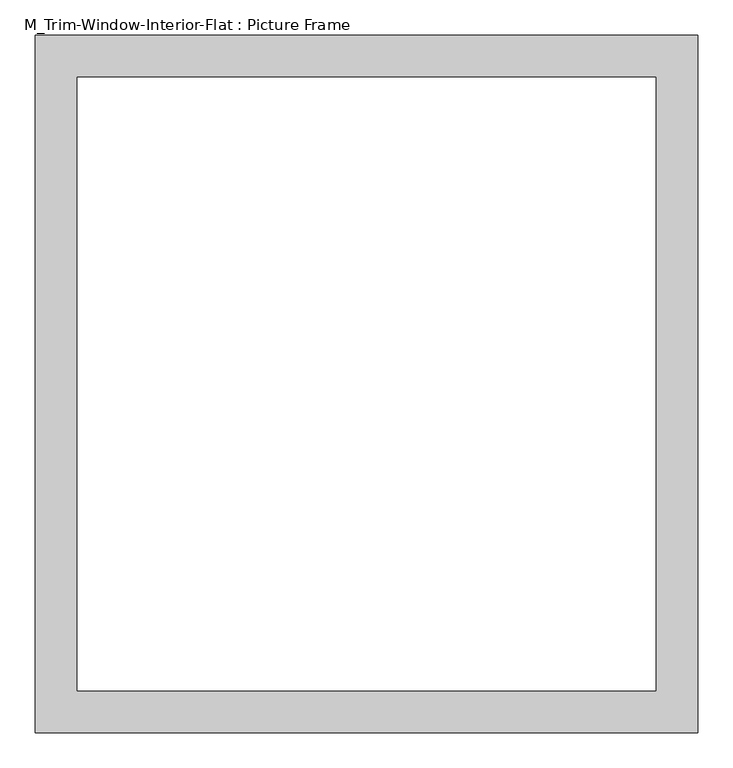
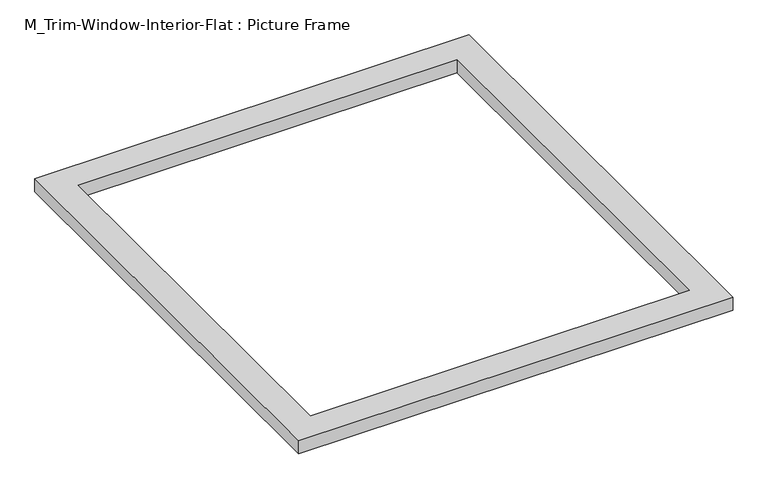
"""IFC4 building model written with IfcOpenShell, lengths in millimetres: proxy geometry, M_Trim-Window-Interior-Flat : Picture Frame."""

from ifc_helpers import new_model, si_unit, origin, origin_with_axes, place, context, project, spatial, polyline, outline, extrude, source, transform, mapped, element, save


def m_trim_window_interior_flat_picture_frame_8dc44e6e(model_context):
    return source(origin(), model_context, "Body", "SweptSolid", [
        extrude(outline(polyline([(472.3, -47.3), (-472.3, -47.3), (-472.3, 947.3), (472.3, 947.3), (472.3, -47.3)]), holes=[polyline([(412.3, 12.7), (412.3, 887.3), (-412.3, 887.3), (-412.3, 12.7), (412.3, 12.7)])]), origin_with_axes(), (0.0, 0.0, 1.0), 30.0),
    ])


if __name__ == "__main__":
    model = new_model("IFC4")
    model_context = context("Model", 3, world=origin())
    ifc_project = project(units=[si_unit("LENGTHUNIT", "METRE", prefix="MILLI")], contexts=[model_context])
    site = spatial("IfcSite", under=ifc_project)
    building = spatial("IfcBuilding", under=site)
    placement = place(None, origin())
    m_trim_window_interior_flat_picture_frame_shape = m_trim_window_interior_flat_picture_frame_8dc44e6e(model_context)
    element("IfcBuildingElementProxy", 1, Name="M_Trim-Window-Interior-Flat : Picture Frame", ObjectType="M_Trim-Window-Interior-Flat : Picture Frame", at=placement, inside=building, context=model_context, shape_type="MappedRepresentation", body=[
        mapped(m_trim_window_interior_flat_picture_frame_shape, transform((0.0, 0.0, 0.0), x_axis=(1.0, 0.0, 0.0), y_axis=(0.0, 1.0, 0.0), z_axis=(0.0, 0.0, 1.0))),
    ])
    save(model, "model.ifc")

# Revit data of these elements
# Type "M_Trim-Window-Interior-Flat : Picture Frame"
#   Trim Thickness_Picture Frame = 30 mm
#   Trim Width = 60 mm
#   Trim Thickness_with Sill = 20 mm
#   Sill Thickness = 30 mm
#   Opening Width [instance default] = 600 mm
#   Opening Height [instance default] = 900 mm
#   Default Elevation = 1200 mm
#   Sill = no
#   Picture Frame = yes
#   Trim Material [instance default] = none
# Element 1 (IfcBuildingElementProxy, "M_Trim-Window-Interior-Flat : Picture Frame")
#   Opening Width = 850 mm
#   Trim Material = Wood - Stained
#   Materials on its faces: "Wood - Stained"
# Materials
#   "Wood - Stained": class "Wood", colour RGB 224 178 126, transparency 0, Cost = 0
